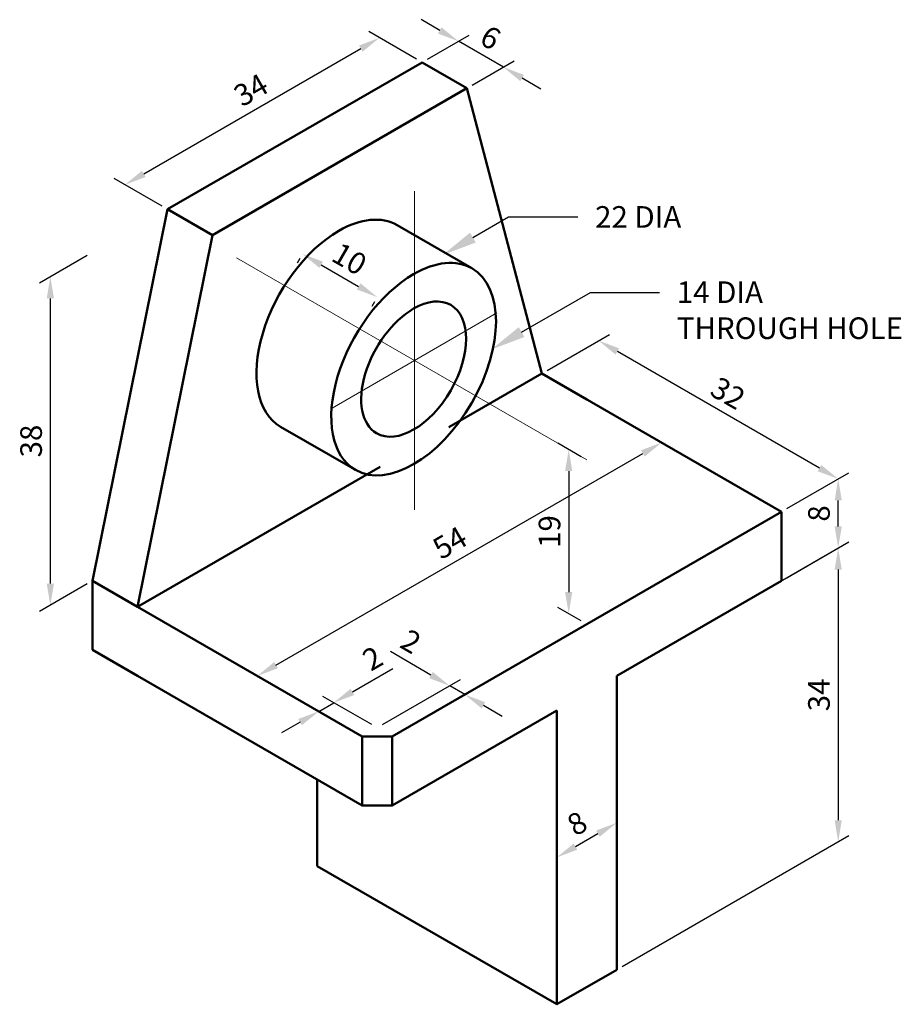
# Model space of a CAD drawing. Units: millimetres. Extents: x 1894 to 1996, y 1268 to 1382.
import ezdxf
from ezdxf import colors
from ezdxf.entities.mleader import LeaderData, LeaderLine
from ezdxf.math import Vec2, Vec3

# ---------------------------------------------------------------- set-up
doc = ezdxf.new("R2010")
doc.units = ezdxf.units.MM
doc.linetypes.add('CENTER', pattern=[50.8, 31.75, -6.35, 6.35, -6.35])
for name, color, linetype, lineweight in [('M-CNTR', 4, 'CENTER', 18), ('M-DIMS', 2, 'Continuous', 25), ('M-OUTL', 7, 'Continuous', 50)]:
    doc.layers.add(name, color=color, linetype=linetype, lineweight=lineweight)
doc.styles.get("Standard").update_dxf_attribs({"font": 'arial.ttf'})
doc.dimstyles.new('ISO-25', dxfattribs={"dimtxt": 2.5, "dimasz": 2.5, "dimexe": 1.25, "dimexo": 0.625, "dimtad": 1, "dimtxsty": 'Standard', "dimcen": 2.5, "dimadec": 0, "dimazin": 0, "dimtfac": 1, "dimtmove": 0, "dimatfit": 3, "dimfxl": 1, "dimarcsym": 0})

# ---------------------------------------------------------------- blocks, each defined once
blk = doc.blocks.new('*D1')
at = {"layer": 'Defpoints', "color": 0, "transparency": 16777216}
for p in [(1902.87, 1354.6), (1902.87, 1316.6), (1897.98, 1313.78)]:
    blk.add_point(p, dxfattribs=at)
at = {"layer": 'M-DIMS', "color": 0, "lineweight": -2, "transparency": 16777216}
for p, q in [((1902.24, 1354.24), (1896.73, 1351.06)), ((1897.98, 1349.28), (1897.98, 1316.28)), ((1902.24, 1316.24), (1896.73, 1313.06))]:
    blk.add_line(p, q, dxfattribs=at)
at = {"layer": 'M-DIMS', "color": 0, "transparency": 16777216}
for points in [[(1897.56, 1349.28), (1898.4, 1349.28), (1897.98, 1351.78)], [(1897.56, 1316.28), (1898.4, 1316.28), (1897.98, 1313.78)]]:
    blk.add_solid(points, dxfattribs=at)
at = {"layer": 'M-DIMS', "color": 0, "transparency": 16777216, "insert": (1896.08, 1332.78), "char_height": 2.5, "attachment_point": 5, "rotation": 90}
blk.add_mtext('38', dxfattribs=at)
blk = doc.blocks.new('*D2')
at = {"layer": 'Defpoints', "color": 0, "transparency": 16777216}
for p in [(1963.49, 1305.6), (1989.11, 1286.4), (1963.49, 1271.6)]:
    blk.add_point(p, dxfattribs=at)
at = {"layer": 'M-DIMS', "color": 0, "lineweight": -2, "transparency": 16777216}
for p, q in [((1964.11, 1305.96), (1990.36, 1321.12)), ((1989.11, 1317.9), (1989.11, 1288.9)), ((1964.11, 1271.96), (1990.36, 1287.12))]:
    blk.add_line(p, q, dxfattribs=at)
at = {"layer": 'M-DIMS', "color": 0, "transparency": 16777216}
for points in [[(1988.7, 1317.9), (1989.53, 1317.9), (1989.11, 1320.4)], [(1988.7, 1288.9), (1989.53, 1288.9), (1989.11, 1286.4)]]:
    blk.add_solid(points, dxfattribs=at)
at = {"layer": 'M-DIMS', "color": 0, "transparency": 16777216, "insert": (1987.21, 1303.4), "char_height": 2.5, "attachment_point": 5, "rotation": 90}
blk.add_mtext('34', dxfattribs=at)
blk = doc.blocks.new('*D3')
at = {"layer": 'Defpoints', "color": 0, "transparency": 16777216}
for p in [(1989.11, 1328.4), (1982.54, 1324.6), (1982.54, 1316.6)]:
    blk.add_point(p, dxfattribs=at)
at = {"layer": 'M-DIMS', "color": 0, "lineweight": -2, "transparency": 16777216}
for p, q in [((1983.17, 1324.96), (1990.36, 1329.12)), ((1989.11, 1322.9), (1989.11, 1325.9)), ((1983.17, 1316.96), (1990.36, 1321.12))]:
    blk.add_line(p, q, dxfattribs=at)
at = {"layer": 'M-DIMS', "color": 0, "transparency": 16777216}
for points in [[(1988.7, 1325.9), (1989.53, 1325.9), (1989.11, 1328.4)], [(1988.7, 1322.9), (1989.53, 1322.9), (1989.11, 1320.4)]]:
    blk.add_solid(points, dxfattribs=at)
at = {"layer": 'M-DIMS', "color": 0, "transparency": 16777216, "insert": (1987.21, 1324.4), "char_height": 2.5, "attachment_point": 5, "rotation": 90}
blk.add_mtext('8', dxfattribs=at)
blk = doc.blocks.new('*D4')
at = {"layer": 'Defpoints', "color": 0, "transparency": 16777216}
for p in [(1961.4, 1344.4), (1954.83, 1340.6), (1982.54, 1324.6)]:
    blk.add_point(p, dxfattribs=at)
at = {"layer": 'M-DIMS', "color": 0, "lineweight": -2, "transparency": 16777216}
for p, q in [((1955.45, 1340.96), (1962.65, 1345.12)), ((1986.95, 1329.65), (1963.57, 1343.15)), ((1983.17, 1324.96), (1990.36, 1329.12))]:
    blk.add_line(p, q, dxfattribs=at)
at = {"layer": 'M-DIMS', "color": 0, "transparency": 16777216}
for points in [[(1963.77, 1343.51), (1963.36, 1342.78), (1961.4, 1344.4)], [(1987.16, 1330.01), (1986.74, 1329.28), (1989.11, 1328.4)]]:
    blk.add_solid(points, dxfattribs=at)
at = {"layer": 'M-DIMS', "color": 0, "transparency": 16777216, "insert": (1976.21, 1338.04), "char_height": 2.5, "attachment_point": 5, "rotation": 330}
blk.add_mtext('32', dxfattribs=at)
blk = doc.blocks.new('*D5')
at = {"layer": 'Defpoints', "color": 0, "transparency": 16777216}
for p in [(1963.49, 1305.6), (1956.56, 1301.6), (1963.49, 1288.6)]:
    blk.add_point(p, dxfattribs=at)
at = {"layer": 'M-DIMS', "color": 0, "lineweight": -2, "transparency": 16777216}
for p, q in [((1963.49, 1304.88), (1963.49, 1287.16)), ((1956.56, 1300.88), (1956.56, 1283.16)), ((1958.72, 1285.85), (1961.32, 1287.35))]:
    blk.add_line(p, q, dxfattribs=at)
at = {"layer": 'M-DIMS', "color": 0, "transparency": 16777216}
for points in [[(1961.11, 1287.71), (1961.53, 1286.99), (1963.49, 1288.6)], [(1958.52, 1286.21), (1958.93, 1285.49), (1956.56, 1284.6)]]:
    blk.add_solid(points, dxfattribs=at)
at = {"layer": 'M-DIMS', "color": 0, "transparency": 16777216, "insert": (1959.07, 1288.25), "char_height": 2.5, "attachment_point": 5, "rotation": 30}
blk.add_mtext('8', dxfattribs=at)
blk = doc.blocks.new('*D6')
at = {"layer": 'Defpoints', "color": 0, "transparency": 16777216}
for p in [(1936.06, 1379.44), (1940.97, 1376.6), (1911.53, 1359.6)]:
    blk.add_point(p, dxfattribs=at)
at = {"layer": 'M-DIMS', "color": 0, "lineweight": -2, "transparency": 16777216}
for p, q in [((1940.35, 1376.96), (1934.81, 1380.16)), ((1908.78, 1363.69), (1933.9, 1378.19)), ((1910.9, 1359.96), (1905.37, 1363.16))]:
    blk.add_line(p, q, dxfattribs=at)
at = {"layer": 'M-DIMS', "color": 0, "transparency": 16777216}
for points in [[(1933.69, 1378.55), (1934.1, 1377.83), (1936.06, 1379.44)], [(1908.57, 1364.05), (1908.99, 1363.33), (1906.62, 1362.44)]]:
    blk.add_solid(points, dxfattribs=at)
at = {"layer": 'M-DIMS', "color": 0, "transparency": 16777216, "insert": (1921.34, 1373.13), "char_height": 2.5, "attachment_point": 5, "rotation": 30}
blk.add_mtext('34', dxfattribs=at)
blk = doc.blocks.new('*D7')
at = {"layer": 'Defpoints', "color": 0, "transparency": 16777216}
for p in [(1954.83, 1340.6), (1968.68, 1332.6), (1908.06, 1313.6)]:
    blk.add_point(p, dxfattribs=at)
at = {"layer": 'M-DIMS', "color": 0, "lineweight": -2, "transparency": 16777216}
for p, q in [((1955.45, 1340.24), (1969.93, 1331.88)), ((1924.08, 1306.85), (1966.52, 1331.35)), ((1908.69, 1313.24), (1923.17, 1304.88))]:
    blk.add_line(p, q, dxfattribs=at)
at = {"layer": 'M-DIMS', "color": 0, "transparency": 16777216}
for points in [[(1966.31, 1331.71), (1966.73, 1330.99), (1968.68, 1332.6)], [(1923.88, 1307.21), (1924.29, 1306.49), (1921.92, 1305.6)]]:
    blk.add_solid(points, dxfattribs=at)
at = {"layer": 'M-DIMS', "color": 0, "transparency": 16777216, "insert": (1944.35, 1320.74), "char_height": 2.5, "attachment_point": 5, "rotation": 30}
blk.add_mtext('54', dxfattribs=at)
blk = doc.blocks.new('*D8')
at = {"layer": 'Defpoints', "color": 0, "transparency": 16777216}
for p in [(1945.19, 1379.04), (1940.97, 1376.6), (1946.17, 1373.6)]:
    blk.add_point(p, dxfattribs=at)
at = {"layer": 'M-DIMS', "color": 0, "lineweight": -2, "transparency": 16777216}
for p, q in [((1943.02, 1380.29), (1940.86, 1381.54)), ((1941.6, 1376.96), (1946.44, 1379.76)), ((1950.39, 1376.04), (1945.19, 1379.04)), ((1946.79, 1373.96), (1951.64, 1376.76)), ((1952.55, 1374.79), (1954.72, 1373.54))]:
    blk.add_line(p, q, dxfattribs=at)
at = {"layer": 'M-DIMS', "color": 0, "transparency": 16777216}
for points in [[(1943.23, 1380.65), (1942.82, 1379.93), (1945.19, 1379.04)], [(1952.76, 1375.15), (1952.34, 1374.43), (1950.39, 1376.04)]]:
    blk.add_solid(points, dxfattribs=at)
at = {"layer": 'M-DIMS', "color": 0, "transparency": 16777216, "insert": (1948.74, 1379.18), "char_height": 2.5, "attachment_point": 5, "rotation": 330}
blk.add_mtext('6', dxfattribs=at)
blk = doc.blocks.new('*D9')
at = {"layer": 'Defpoints', "color": 0, "transparency": 16777216}
for p in [(1930.76, 1302.5), (1935.77, 1299.6), (1934.04, 1298.6)]:
    blk.add_point(p, dxfattribs=at)
at = {"layer": 'M-DIMS', "color": 0, "lineweight": -2, "transparency": 16777216}
for p, q in [((1932.93, 1303.75), (1937.61, 1306.45)), ((1929.03, 1301.5), (1930.76, 1302.5)), ((1935.15, 1299.96), (1929.51, 1303.22)), ((1933.42, 1298.96), (1927.78, 1302.22)), ((1926.86, 1300.25), (1924.7, 1299))]:
    blk.add_line(p, q, dxfattribs=at)
at = {"layer": 'M-DIMS', "color": 0, "transparency": 16777216}
for points in [[(1932.72, 1304.11), (1933.13, 1303.39), (1930.76, 1302.5)], [(1926.65, 1300.61), (1927.07, 1299.89), (1929.03, 1301.5)]]:
    blk.add_solid(points, dxfattribs=at)
at = {"layer": 'M-DIMS', "color": 0, "transparency": 16777216, "insert": (1935.41, 1307.35), "char_height": 2.5, "attachment_point": 5, "rotation": 30}
blk.add_mtext('2', dxfattribs=at)
blk = doc.blocks.new('*D10')
at = {"layer": 'Defpoints', "color": 0, "transparency": 16777216}
for p in [(1944.18, 1304.45), (1935.77, 1299.6), (1937.51, 1298.6)]:
    blk.add_point(p, dxfattribs=at)
at = {"layer": 'M-DIMS', "color": 0, "lineweight": -2, "transparency": 16777216}
for p, q in [((1942.01, 1305.7), (1937.33, 1308.41)), ((1936.4, 1299.96), (1945.43, 1305.17)), ((1938.13, 1298.96), (1947.16, 1304.17)), ((1945.91, 1303.45), (1944.18, 1304.45)), ((1948.08, 1302.2), (1950.24, 1300.95))]:
    blk.add_line(p, q, dxfattribs=at)
at = {"layer": 'M-DIMS', "color": 0, "transparency": 16777216}
for points in [[(1942.22, 1306.06), (1941.8, 1305.34), (1944.18, 1304.45)], [(1948.28, 1302.56), (1947.87, 1301.84), (1945.91, 1303.45)]]:
    blk.add_solid(points, dxfattribs=at)
at = {"layer": 'M-DIMS', "color": 0, "transparency": 16777216, "insert": (1939.53, 1309.31), "char_height": 2.5, "attachment_point": 5, "rotation": 330}
blk.add_mtext('2', dxfattribs=at)
blk = doc.blocks.new('*D11')
at = {"layer": 'Defpoints', "color": 0, "transparency": 16777216}
for p in [(1960.02, 1330.6), (1957.94, 1312.81), (1960.02, 1311.6)]:
    blk.add_point(p, dxfattribs=at)
at = {"layer": 'M-DIMS', "color": 0, "lineweight": -2, "transparency": 16777216}
for p, q in [((1959.4, 1330.96), (1956.69, 1332.53)), ((1957.94, 1329.31), (1957.94, 1315.31)), ((1959.4, 1311.96), (1956.69, 1313.53))]:
    blk.add_line(p, q, dxfattribs=at)
at = {"layer": 'M-DIMS', "color": 0, "transparency": 16777216}
for points in [[(1957.52, 1329.31), (1958.35, 1329.31), (1957.94, 1331.81)], [(1957.52, 1315.31), (1958.35, 1315.31), (1957.94, 1312.81)]]:
    blk.add_solid(points, dxfattribs=at)
at = {"layer": 'M-DIMS', "color": 0, "transparency": 16777216, "insert": (1956.04, 1322.31), "char_height": 2.5, "attachment_point": 5, "rotation": 90}
blk.add_mtext('19', dxfattribs=at)
blk = doc.blocks.new('*D12')
at = {"layer": 'Defpoints', "color": 0, "transparency": 16777216}
for p in [(1927.14, 1354.43), (1935.8, 1349.43), (1935.8, 1349.43)]:
    blk.add_point(p, dxfattribs=at)
at = {"layer": 'M-DIMS', "color": 0, "lineweight": -2, "transparency": 16777216}
for p, q in [((1926.83, 1353.89), (1926.52, 1353.35)), ((1929.31, 1353.18), (1933.64, 1350.68)), ((1935.49, 1348.89), (1935.18, 1348.35))]:
    blk.add_line(p, q, dxfattribs=at)
at = {"layer": 'M-DIMS', "color": 0, "transparency": 16777216}
for points in [[(1929.51, 1353.54), (1929.1, 1352.82), (1927.14, 1354.43)], [(1933.85, 1351.04), (1933.43, 1350.32), (1935.8, 1349.43)]]:
    blk.add_solid(points, dxfattribs=at)
at = {"layer": 'M-DIMS', "color": 0, "transparency": 16777216, "insert": (1932.42, 1353.58), "char_height": 2.5, "attachment_point": 5, "rotation": 330}
blk.add_mtext('10', dxfattribs=at)

msp = doc.modelspace()

# ---------------------------------------------------------------- linework, layer by layer
at = {"layer": 'M-CNTR'}
for p, q in [((1940.105, 1342.101), (1940.105, 1361.704)), ((1940.105, 1342.101), (1919.527, 1353.982)), ((1940.105, 1342.101), (1949.631, 1347.601)), ((1940.105, 1342.101), (1930.579, 1336.601)), ((1940.105, 1342.101), (1956.599, 1332.578)), ((1940.105, 1342.101), (1940.105, 1324.809)), ((1956.599, 1332.578), (1960.024, 1330.601))]:
    msp.add_line(p, q, dxfattribs=at)
at = {"layer": 'M-OUTL'}
for p, q in [((1926.249, 1368.101), (1940.971, 1376.601)), ((1940.971, 1376.601), (1946.167, 1373.601)), ((1916.722, 1356.601), (1946.167, 1373.601)), ((1946.167, 1373.601), (1954.827, 1340.601)), ((1926.249, 1368.101), (1911.526, 1359.601)), ((1911.526, 1359.601), (1902.866, 1316.601)), ((1911.526, 1359.601), (1916.722, 1356.601)), ((1946.741, 1352.768), (1938.081, 1357.768)), ((1916.722, 1356.601), (1908.062, 1313.601)), ((1944.074, 1334.392), (1954.827, 1340.601)), ((1982.54, 1324.601), (1954.827, 1340.601)), ((1954.827, 1340.601), (1960.024, 1337.601)), ((1933.269, 1329.434), (1924.609, 1334.434)), ((1908.062, 1313.601), (1936.136, 1329.81)), ((1937.507, 1298.601), (1982.54, 1324.601)), ((1982.54, 1324.601), (1982.54, 1316.601)), ((1908.062, 1313.601), (1902.866, 1316.601)), ((1902.866, 1316.601), (1902.866, 1308.601)), ((1982.54, 1316.601), (1963.488, 1305.601)), ((1934.043, 1298.601), (1908.062, 1313.601)), ((1902.866, 1308.601), (1908.062, 1305.601)), ((1908.062, 1305.601), (1934.043, 1290.601)), ((1963.488, 1305.601), (1963.488, 1271.601)), ((1956.56, 1301.601), (1937.507, 1290.601)), ((1956.56, 1301.601), (1956.56, 1267.601)), ((1934.043, 1298.601), (1937.507, 1298.601)), ((1934.043, 1298.601), (1934.043, 1290.601)), ((1937.507, 1298.601), (1937.507, 1290.601)), ((1928.847, 1283.601), (1928.847, 1293.601)), ((1934.043, 1290.601), (1937.507, 1290.601)), ((1956.56, 1267.601), (1928.847, 1283.601)), ((1963.488, 1271.601), (1956.56, 1267.601))]:
    msp.add_line(p, q, dxfattribs=at)
for centre, major_axis, start_param, end_param in [((1931.345, 1346.101), (6.736, 11.667), 0, 0.7853982), ((1931.345, 1346.101), (6.736, 11.667), 0.7853982, 3.1415927), ((1940.005, 1341.101), (6.736, 11.667), 0, 0.7853982), ((1940.005, 1341.101), (6.736, 11.667), 3.1415927, 6.2831853), ((1940.005, 1341.101), (6.736, 11.667), 0.7853982, 3.1415927), ((1940.005, 1341.101), (4.287, 7.425), 0, 0.7853982), ((1940.005, 1341.101), (4.287, 7.425), 0.7853982, 3.1415927), ((1940.005, 1341.101), (4.287, 7.425), 3.1415927, 6.2831853)]:
    msp.add_ellipse(centre, major_axis=major_axis, ratio=0.5773503, start_param=start_param, end_param=end_param, dxfattribs=at)

# ---------------------------------------------------------------- dimensions: what is measured, and where the dimension line sits
at = {"layer": 'M-DIMS'}
for base, p1, p2, angle, picture, middle in [((1945.19, 1379.037), (1946.167, 1373.601), (1940.971, 1376.601), 150, '*D8', (1947.788, 1377.537)), ((1936.061, 1379.436), (1911.526, 1359.601), (1940.971, 1376.601), 30, '*D6', (1922.29, 1371.485)), ((1944.178, 1304.453), (1937.507, 1298.601), (1935.775, 1299.601), 150, '*D10', (1938.59, 1307.679)), ((1930.76, 1302.496), (1934.043, 1298.601), (1935.775, 1299.601), 30, '*D9', (1936.348, 1305.723))]:
    dim = msp.add_linear_dim(base=base, p1=p1, p2=p2, angle=angle, dimstyle='ISO-25', override={"dimclrd": 0, "dimclre": 0, "dimclrt": 0}, dxfattribs=at)
    dim.commit()
    dim.dimension.update_dxf_attribs({"geometry": picture, "text_midpoint": middle, "dimtype": 161})
for p1, p2, distance, picture, middle in [((1927.142, 1354.43), (1935.802, 1349.43), 0, '*D12', (1932.422, 1353.577)), ((1902.866, 1354.601), (1902.866, 1316.601), -4.886, '*D1', (1896.077, 1332.78)), ((1982.54, 1324.601), (1954.827, 1340.601), -6.573, '*D4', (1976.208, 1338.043)), ((1908.062, 1313.601), (1954.827, 1340.601), -13.856, '*D7', (1944.353, 1320.743)), ((1960.024, 1330.601), (1960.024, 1311.601), -2.087, '*D11', (1956.036, 1322.306)), ((1982.54, 1316.601), (1982.54, 1324.601), -6.573, '*D3', (1987.212, 1324.396)), ((1963.488, 1305.601), (1963.488, 1271.601), 25.625, '*D2', (1987.211, 1303.396)), ((1956.56, 1301.601), (1963.488, 1305.601), -14.722, '*D5', (1959.073, 1288.248))]:
    dim = msp.add_aligned_dim(p1=p1, p2=p2, distance=distance, dimstyle='ISO-25', override={"dimclrd": 0, "dimclre": 0, "dimclrt": 0}, dxfattribs=at)
    dim.commit()
    dim.dimension.update_dxf_attribs({"geometry": picture, "text_midpoint": middle})

# ---------------------------------------------------------------- leaders
ml = msp.add_multileader_mtext('Standard', dxfattribs=at)
ml.set_content('22 DIA', color=256)
ml.set_leader_properties()
ml.build(insert=Vec2(0, 0))
ctx = ml.context
ctx.base_point, ctx.char_height, ctx.plane_origin = Vec3(1958.992, 1358.71), 2.5, Vec3(1943.393, 1354.323)
notes = []
notes.append((ctx, [(0, (1, 1, 0), (1950.992, 1358.71), (1, 0), 8, [(0, [(1943.393, 1354.323)], 0, [])])]))
ctx.mtext.insert, ctx.mtext.flow_direction = Vec3(1960.992, 1359.961), 5
ml = msp.add_multileader_mtext('Standard', dxfattribs=at)
ml.set_content('14 DIA\\PTHROUGH HOLE', color=256)
ml.set_leader_properties()
ml.build(insert=Vec2(0, 0))
ctx = ml.context
ctx.base_point, ctx.char_height, ctx.plane_origin = Vec3(1968.446, 1349.981), 2.5, Vec3(1949.024, 1343.387)
notes.append((ctx, [(0, (1, 1, 0), (1960.446, 1349.981), (1, 0), 8, [(0, [(1949.024, 1343.387)], 0, [])])]))
ctx.mtext.insert, ctx.mtext.flow_direction = Vec3(1970.446, 1351.253), 5
for ctx, leaders in notes:
    for number, flags, end, landing, length, lines in leaders:
        leader = LeaderData()
        leader.index, (leader.has_last_leader_line, leader.has_dogleg_vector, leader.attachment_direction) = number, flags
        leader.last_leader_point, leader.dogleg_vector, leader.dogleg_length = Vec3(end), Vec3(landing), length
        for number, points, colour, breaks in lines:
            line = LeaderLine()
            line.index, line.vertices, line.color, line.breaks = number, Vec3.list(points), colors.encode_raw_color(colour), breaks
            leader.lines.append(line)
        ctx.leaders.append(leader)

doc.saveas('drawing.dxf')
